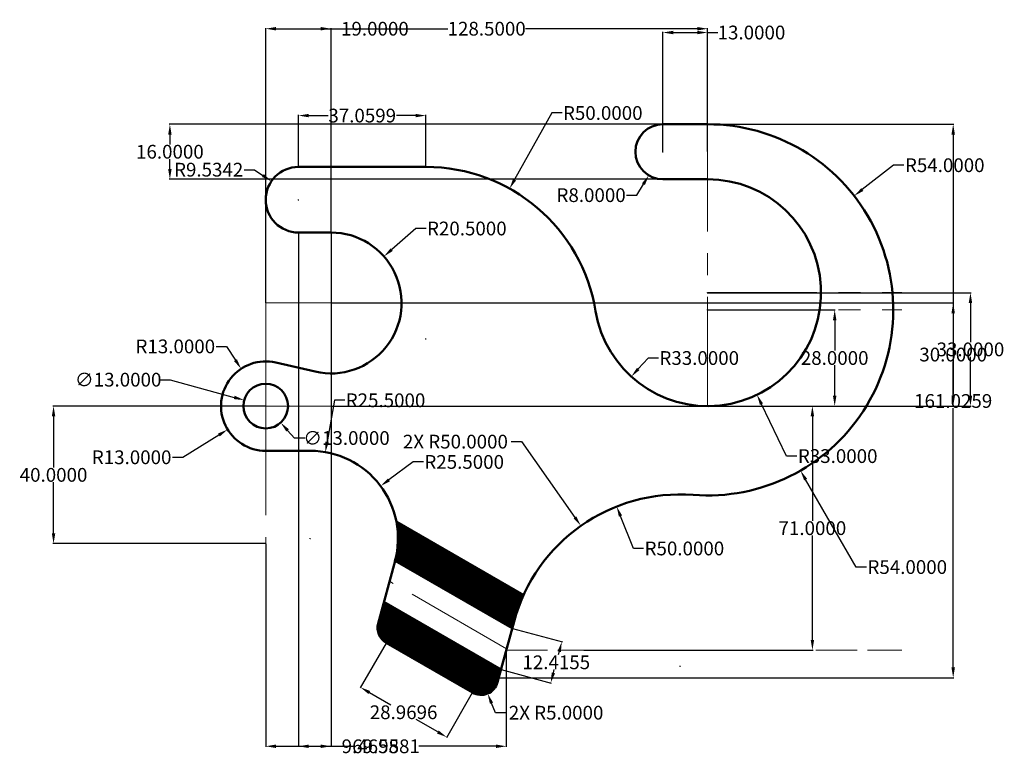
# Model space of a CAD drawing. Units: millimetres. Extents: x 855 to 1141, y 767 to 981.
import ezdxf

# ---------------------------------------------------------------- set-up
doc = ezdxf.new("R2010")
doc.units = ezdxf.units.MM
doc.header["$MEASUREMENT"] = 0
doc.linetypes.add('ACAD_ISO02W100', pattern=[15, 12, -3])
doc.linetypes.add('CENTER', pattern=[50.8, 31.75, -6.35, 6.35, -6.35])
for name, color, linetype, lineweight in [('M-CNTR', 55, 'CENTER', 18), ('M-CONS', 2, 'ACAD_ISO02W100', 13), ('M-DIMS', 2, 'Continuous', 25), ('M-HATC', 8, 'Continuous', 18), ('M-OUTL', 7, 'Continuous', 50)]:
    doc.layers.add(name, color=color, linetype=linetype, lineweight=lineweight)
doc.styles.get("Standard").update_dxf_attribs({"font": 'arial.ttf'})
doc.dimstyles.get("Standard").update_dxf_attribs({"dimtxt": 4, "dimasz": 3, "dimexe": 0.18, "dimexo": 0.0625, "dimgap": 0.09, "dimtad": 0, "dimtih": 1, "dimtoh": 1, "dimdec": 4, "dimzin": 0, "dimdsep": 46, "dimtxsty": 'Standard', "dimcen": 0.09, "dimadec": 0, "dimazin": 0, "dimtfac": 1, "dimtdec": 4, "dimtofl": 0, "dimtmove": 0, "dimatfit": 3, "dimfxl": 1, "dimtolj": 1, "dimtzin": 0, "dimarcsym": 0})

# ---------------------------------------------------------------- blocks, each defined once
blk = doc.blocks.new('*D1')
at = {"layer": 'Defpoints', "color": 0, "transparency": 16777216}
for p in [(1055.15, 901.49), (1032.96, 877.07)]:
    blk.add_point(p, dxfattribs=at)
at = {"layer": 'M-DIMS', "color": 0, "lineweight": -2, "transparency": 16777216}
for p, q in [((1037.87, 882.48), (1034.97, 879.29)), ((1040.87, 882.48), (1037.87, 882.48))]:
    blk.add_line(p, q, dxfattribs=at)
at = {"layer": 'M-DIMS', "color": 0, "transparency": 16777216}
blk.add_solid([(1034.6, 879.63), (1035.34, 878.96), (1032.96, 877.07)], dxfattribs=at)
at = {"layer": 'M-DIMS', "color": 0, "transparency": 16777216, "insert": (1052.72, 882.48), "char_height": 4, "attachment_point": 5}
blk.add_mtext('\\A1;R33.0000', dxfattribs=at)
blk = doc.blocks.new('*D2')
at = {"layer": 'Defpoints', "color": 0, "transparency": 16777216}
for p in [(997.56, 931.75), (973.24, 888.06)]:
    blk.add_point(p, dxfattribs=at)
at = {"layer": 'M-DIMS', "color": 0, "lineweight": -2, "transparency": 16777216}
for p, q in [((1009.81, 953.76), (999.02, 934.37)), ((1012.81, 953.76), (1009.81, 953.76)), ((973.15, 888.06), (973.33, 888.06)), ((973.24, 887.97), (973.24, 888.15))]:
    blk.add_line(p, q, dxfattribs=at)
at = {"layer": 'M-DIMS', "color": 0, "transparency": 16777216}
blk.add_solid([(998.58, 934.62), (999.46, 934.13), (997.56, 931.75)], dxfattribs=at)
at = {"layer": 'M-DIMS', "color": 0, "transparency": 16777216, "insert": (1024.66, 953.76), "char_height": 4, "attachment_point": 5}
blk.add_mtext('\\A1;R50.0000', dxfattribs=at)
blk = doc.blocks.new('*D3')
at = {"layer": 'Defpoints', "color": 0, "transparency": 16777216}
for p in [(1042.15, 942.49), (1038.03, 935.63)]:
    blk.add_point(p, dxfattribs=at)
at = {"layer": 'M-DIMS', "color": 0, "lineweight": -2, "transparency": 16777216}
for p, q in [((1042.06, 942.49), (1042.24, 942.49)), ((1042.15, 942.4), (1042.15, 942.58)), ((1034.57, 929.86), (1036.49, 933.06)), ((1031.57, 929.86), (1034.57, 929.86))]:
    blk.add_line(p, q, dxfattribs=at)
at = {"layer": 'M-DIMS', "color": 0, "transparency": 16777216}
blk.add_solid([(1036.06, 933.32), (1036.92, 932.8), (1038.03, 935.63)], dxfattribs=at)
at = {"layer": 'M-DIMS', "color": 0, "transparency": 16777216, "insert": (1021.27, 929.86), "char_height": 4, "attachment_point": 5}
blk.add_mtext('\\A1;R8.0000', dxfattribs=at)
blk = doc.blocks.new('*D4')
at = {"layer": 'Defpoints', "color": 0, "transparency": 16777216}
for p in [(926.65, 868.49), (915.58, 861.67)]:
    blk.add_point(p, dxfattribs=at)
at = {"layer": 'M-DIMS', "color": 0, "lineweight": -2, "transparency": 16777216}
for p, q in [((926.56, 868.49), (926.74, 868.49)), ((926.65, 868.4), (926.65, 868.58)), ((902.51, 853.61), (913.03, 860.1)), ((899.51, 853.61), (902.51, 853.61))]:
    blk.add_line(p, q, dxfattribs=at)
at = {"layer": 'M-DIMS', "color": 0, "transparency": 16777216}
blk.add_solid([(912.77, 860.52), (913.29, 859.67), (915.58, 861.67)], dxfattribs=at)
at = {"layer": 'M-DIMS', "color": 0, "transparency": 16777216, "insert": (887.66, 853.61), "char_height": 4, "attachment_point": 5}
blk.add_mtext('\\A1;R13.0000', dxfattribs=at)
blk = doc.blocks.new('*D5')
at = {"layer": 'Defpoints', "color": 0, "transparency": 16777216}
for p in [(920.39, 870.23), (932.92, 866.76)]:
    blk.add_point(p, dxfattribs=at)
at = {"layer": 'M-DIMS', "color": 0, "lineweight": -2, "transparency": 16777216}
for p, q in [((895.85, 876.18), (898.85, 876.18)), ((898.85, 876.18), (917.49, 871.03)), ((926.56, 868.49), (926.74, 868.49)), ((926.65, 868.4), (926.65, 868.58))]:
    blk.add_line(p, q, dxfattribs=at)
at = {"layer": 'M-DIMS', "color": 0, "transparency": 16777216}
blk.add_solid([(917.63, 871.51), (917.36, 870.54), (920.39, 870.23)], dxfattribs=at)
at = {"layer": 'M-DIMS', "color": 0, "transparency": 16777216, "insert": (883.74, 876.18), "char_height": 4, "attachment_point": 5}
blk.add_mtext('\\A1;∅13.0000', dxfattribs=at)
blk = doc.blocks.new('*D6')
at = {"layer": 'Defpoints', "color": 0, "transparency": 16777216}
for p in [(1028.71, 839.28), (1047.14, 792.8)]:
    blk.add_point(p, dxfattribs=at)
at = {"layer": 'M-DIMS', "color": 0, "lineweight": -2, "transparency": 16777216}
for p, q in [((1033.55, 827.08), (1029.82, 836.5)), ((1036.55, 827.08), (1033.55, 827.08))]:
    blk.add_line(p, q, dxfattribs=at)
at = {"layer": 'M-DIMS', "color": 0, "transparency": 16777216}
blk.add_solid([(1030.28, 836.68), (1029.35, 836.31), (1028.71, 839.28)], dxfattribs=at)
at = {"layer": 'M-DIMS', "color": 0, "transparency": 16777216, "insert": (1048.4, 827.08), "char_height": 4, "attachment_point": 5}
blk.add_mtext('\\A1;R50.0000', dxfattribs=at)
blk = doc.blocks.new('*D7')
at = {"layer": 'Defpoints', "color": 0, "transparency": 16777216}
for p in [(960.07, 845.22), (939.62, 829.99)]:
    blk.add_point(p, dxfattribs=at)
at = {"layer": 'M-DIMS', "color": 0, "lineweight": -2, "transparency": 16777216}
for p, q in [((969.51, 852.25), (962.48, 847.02)), ((972.51, 852.25), (969.51, 852.25)), ((939.53, 829.99), (939.71, 829.99)), ((939.62, 829.9), (939.62, 830.08))]:
    blk.add_line(p, q, dxfattribs=at)
at = {"layer": 'M-DIMS', "color": 0, "transparency": 16777216}
blk.add_solid([(962.18, 847.42), (962.77, 846.61), (960.07, 845.22)], dxfattribs=at)
at = {"layer": 'M-DIMS', "color": 0, "transparency": 16777216, "insert": (984.36, 852.25), "char_height": 4, "attachment_point": 5}
blk.add_mtext('\\A1;R25.5000', dxfattribs=at)
blk = doc.blocks.new('*D8')
at = {"layer": 'Defpoints', "color": 0, "transparency": 16777216}
for p in [(1055.15, 901.49), (1055.15, 868.49), (1131.58, 868.49)]:
    blk.add_point(p, dxfattribs=at)
at = {"layer": 'M-DIMS', "color": 0, "lineweight": -2, "transparency": 16777216}
for p, q in [((1055.21, 901.49), (1131.76, 901.49)), ((1131.58, 898.49), (1131.58, 887.13)), ((1131.58, 871.49), (1131.58, 882.86)), ((1055.21, 868.49), (1131.76, 868.49))]:
    blk.add_line(p, q, dxfattribs=at)
at = {"layer": 'M-DIMS', "color": 0, "transparency": 16777216}
for points in [[(1131.08, 898.49), (1132.08, 898.49), (1131.58, 901.49)], [(1131.08, 871.49), (1132.08, 871.49), (1131.58, 868.49)]]:
    blk.add_solid(points, dxfattribs=at)
at = {"layer": 'M-DIMS', "color": 0, "transparency": 16777216, "insert": (1131.58, 884.99), "char_height": 4, "attachment_point": 5}
blk.add_mtext('\\A1;33.0000', dxfattribs=at)
blk = doc.blocks.new('*D9')
at = {"layer": 'Defpoints', "color": 0, "transparency": 16777216}
for p in [(1055.15, 896.49), (1055.15, 868.49), (1092.1, 868.49)]:
    blk.add_point(p, dxfattribs=at)
at = {"layer": 'M-DIMS', "color": 0, "lineweight": -2, "transparency": 16777216}
for p, q in [((1055.21, 896.49), (1092.28, 896.49)), ((1092.1, 893.49), (1092.1, 884.63)), ((1092.1, 871.49), (1092.1, 880.36)), ((1055.21, 868.49), (1092.28, 868.49))]:
    blk.add_line(p, q, dxfattribs=at)
at = {"layer": 'M-DIMS', "color": 0, "transparency": 16777216}
for points in [[(1091.6, 893.49), (1092.6, 893.49), (1092.1, 896.49)], [(1091.6, 871.49), (1092.6, 871.49), (1092.1, 868.49)]]:
    blk.add_solid(points, dxfattribs=at)
at = {"layer": 'M-DIMS', "color": 0, "transparency": 16777216, "insert": (1092.1, 882.49), "char_height": 4, "attachment_point": 5}
blk.add_mtext('\\A1;28.0000', dxfattribs=at)
blk = doc.blocks.new('*D10')
at = {"layer": 'Defpoints', "color": 0, "transparency": 16777216}
for p in [(1097.78, 929.65), (1055.15, 896.49)]:
    blk.add_point(p, dxfattribs=at)
at = {"layer": 'M-DIMS', "color": 0, "lineweight": -2, "transparency": 16777216}
for p, q in [((1109.25, 938.57), (1100.14, 931.49)), ((1112.25, 938.57), (1109.25, 938.57)), ((1055.06, 896.49), (1055.24, 896.49)), ((1055.15, 896.4), (1055.15, 896.58))]:
    blk.add_line(p, q, dxfattribs=at)
at = {"layer": 'M-DIMS', "color": 0, "transparency": 16777216}
blk.add_solid([(1099.84, 931.88), (1100.45, 931.09), (1097.78, 929.65)], dxfattribs=at)
at = {"layer": 'M-DIMS', "color": 0, "transparency": 16777216, "insert": (1124.11, 938.57), "char_height": 4, "attachment_point": 5}
blk.add_mtext('\\A1;R54.0000', dxfattribs=at)
blk = doc.blocks.new('*D11')
at = {"layer": 'Defpoints', "color": 0, "transparency": 16777216}
for p in [(1055.15, 977.17), (1042.15, 942.49), (1055.15, 942.49)]:
    blk.add_point(p, dxfattribs=at)
at = {"layer": 'M-DIMS', "color": 0, "lineweight": -2, "transparency": 16777216}
for p, q in [((1042.15, 942.56), (1042.15, 977.35)), ((1045.15, 977.17), (1052.15, 977.17)), ((1055.15, 942.56), (1055.15, 977.35)), ((1055.15, 977.17), (1058.15, 977.17))]:
    blk.add_line(p, q, dxfattribs=at)
at = {"layer": 'M-DIMS', "color": 0, "transparency": 16777216}
for points in [[(1045.15, 977.67), (1045.15, 976.67), (1042.15, 977.17)], [(1052.15, 977.67), (1052.15, 976.67), (1055.15, 977.17)]]:
    blk.add_solid(points, dxfattribs=at)
at = {"layer": 'M-DIMS', "color": 0, "transparency": 16777216, "insert": (1067.9, 977.17), "char_height": 4, "attachment_point": 5}
blk.add_mtext('\\A1;13.0000', dxfattribs=at)
blk = doc.blocks.new('*D12')
at = {"layer": 'Defpoints', "color": 0, "transparency": 16777216}
for p in [(1019.13, 868.49), (1019.13, 797.49), (1085.62, 797.49)]:
    blk.add_point(p, dxfattribs=at)
at = {"layer": 'M-DIMS', "color": 0, "lineweight": -2, "transparency": 16777216}
for p, q in [((1019.19, 868.49), (1085.8, 868.49)), ((1085.62, 865.49), (1085.62, 835.13)), ((1085.62, 800.49), (1085.62, 830.86)), ((1019.19, 797.49), (1085.8, 797.49))]:
    blk.add_line(p, q, dxfattribs=at)
at = {"layer": 'M-DIMS', "color": 0, "transparency": 16777216}
for points in [[(1085.12, 865.49), (1086.12, 865.49), (1085.62, 868.49)], [(1085.12, 800.49), (1086.12, 800.49), (1085.62, 797.49)]]:
    blk.add_solid(points, dxfattribs=at)
at = {"layer": 'M-DIMS', "color": 0, "transparency": 16777216, "insert": (1085.62, 832.99), "char_height": 4, "attachment_point": 5}
blk.add_mtext('\\A1;71.0000', dxfattribs=at)
blk = doc.blocks.new('*D13')
at = {"layer": 'Defpoints', "color": 0, "transparency": 16777216}
for p in [(926.74, 868.49), (864.95, 828.49), (926.65, 828.49)]:
    blk.add_point(p, dxfattribs=at)
at = {"layer": 'M-DIMS', "color": 0, "lineweight": -2, "transparency": 16777216}
for p, q in [((926.68, 868.49), (864.77, 868.49)), ((864.95, 865.49), (864.95, 850.63)), ((864.95, 831.49), (864.95, 846.36)), ((926.59, 828.49), (864.77, 828.49))]:
    blk.add_line(p, q, dxfattribs=at)
at = {"layer": 'M-DIMS', "color": 0, "transparency": 16777216}
for points in [[(864.45, 865.49), (865.45, 865.49), (864.95, 868.49)], [(864.45, 831.49), (865.45, 831.49), (864.95, 828.49)]]:
    blk.add_solid(points, dxfattribs=at)
at = {"layer": 'M-DIMS', "color": 0, "transparency": 16777216, "insert": (864.95, 848.49), "char_height": 4, "attachment_point": 5}
blk.add_mtext('\\A1;40.0000', dxfattribs=at)
blk = doc.blocks.new('*D14')
at = {"layer": 'Defpoints', "color": 0, "transparency": 16777216}
for p in [(1055.15, 978.28), (1055.15, 950.49), (926.65, 898.49)]:
    blk.add_point(p, dxfattribs=at)
at = {"layer": 'M-DIMS', "color": 0, "lineweight": -2, "transparency": 16777216}
for p, q in [((926.65, 898.56), (926.65, 978.46)), ((929.65, 978.28), (979.59, 978.28)), ((1052.15, 978.28), (1002.21, 978.28)), ((1055.15, 950.56), (1055.15, 978.46))]:
    blk.add_line(p, q, dxfattribs=at)
at = {"layer": 'M-DIMS', "color": 0, "transparency": 16777216}
for points in [[(929.65, 978.78), (929.65, 977.78), (926.65, 978.28)], [(1052.15, 978.78), (1052.15, 977.78), (1055.15, 978.28)]]:
    blk.add_solid(points, dxfattribs=at)
at = {"layer": 'M-DIMS', "color": 0, "transparency": 16777216, "insert": (990.9, 978.28), "char_height": 4, "attachment_point": 5}
blk.add_mtext('\\A1;128.5000', dxfattribs=at)
blk = doc.blocks.new('*D15')
at = {"layer": 'Defpoints', "color": 0, "transparency": 16777216}
for p in [(1055.15, 950.49), (1126.56, 950.49), (989.26, 789.47)]:
    blk.add_point(p, dxfattribs=at)
at = {"layer": 'M-DIMS', "color": 0, "lineweight": -2, "transparency": 16777216}
for p, q in [((1055.21, 950.49), (1126.74, 950.49)), ((1126.56, 947.49), (1126.56, 872.11)), ((1126.56, 792.47), (1126.56, 867.85)), ((989.32, 789.47), (1126.74, 789.47))]:
    blk.add_line(p, q, dxfattribs=at)
at = {"layer": 'M-DIMS', "color": 0, "transparency": 16777216}
for points in [[(1126.06, 947.49), (1127.06, 947.49), (1126.56, 950.49)], [(1126.06, 792.47), (1127.06, 792.47), (1126.56, 789.47)]]:
    blk.add_solid(points, dxfattribs=at)
at = {"layer": 'M-DIMS', "color": 0, "transparency": 16777216, "insert": (1126.56, 869.98), "char_height": 4, "attachment_point": 5}
blk.add_mtext('\\A1;161.0259', dxfattribs=at)
blk = doc.blocks.new('*D16')
at = {"layer": 'Defpoints', "color": 0, "transparency": 16777216}
for p in [(945.65, 978.28), (945.65, 918.99), (926.65, 898.49)]:
    blk.add_point(p, dxfattribs=at)
at = {"layer": 'M-DIMS', "color": 0, "lineweight": -2, "transparency": 16777216}
for p, q in [((926.65, 898.56), (926.65, 978.46)), ((929.65, 978.28), (942.65, 978.28)), ((945.65, 919.06), (945.65, 978.46)), ((945.65, 978.28), (948.65, 978.28))]:
    blk.add_line(p, q, dxfattribs=at)
at = {"layer": 'M-DIMS', "color": 0, "transparency": 16777216}
for points in [[(929.65, 978.78), (929.65, 977.78), (926.65, 978.28)], [(942.65, 978.78), (942.65, 977.78), (945.65, 978.28)]]:
    blk.add_solid(points, dxfattribs=at)
at = {"layer": 'M-DIMS', "color": 0, "transparency": 16777216, "insert": (958.4, 978.28), "char_height": 4, "attachment_point": 5}
blk.add_mtext('\\A1;19.0000', dxfattribs=at)
blk = doc.blocks.new('*D17')
at = {"layer": 'Defpoints', "color": 0, "transparency": 16777216}
for p in [(945.65, 898.49), (1126.56, 898.49), (945.65, 868.49)]:
    blk.add_point(p, dxfattribs=at)
at = {"layer": 'M-DIMS', "color": 0, "lineweight": -2, "transparency": 16777216}
for p, q in [((945.71, 898.49), (1126.74, 898.49)), ((1126.56, 895.49), (1126.56, 885.63)), ((1126.56, 871.49), (1126.56, 881.36)), ((945.71, 868.49), (1126.74, 868.49))]:
    blk.add_line(p, q, dxfattribs=at)
at = {"layer": 'M-DIMS', "color": 0, "transparency": 16777216}
for points in [[(1126.06, 895.49), (1127.06, 895.49), (1126.56, 898.49)], [(1126.06, 871.49), (1127.06, 871.49), (1126.56, 868.49)]]:
    blk.add_solid(points, dxfattribs=at)
at = {"layer": 'M-DIMS', "color": 0, "transparency": 16777216, "insert": (1126.56, 883.49), "char_height": 4, "attachment_point": 5}
blk.add_mtext('\\A1;30.0000', dxfattribs=at)
blk = doc.blocks.new('*D18')
at = {"layer": 'Defpoints', "color": 0, "transparency": 16777216}
for p in [(898.78, 950.49), (1042.15, 950.49), (1042.15, 934.49)]:
    blk.add_point(p, dxfattribs=at)
at = {"layer": 'M-DIMS', "color": 0, "lineweight": -2, "transparency": 16777216}
for p, q in [((1042.09, 950.49), (898.6, 950.49)), ((898.78, 947.49), (898.78, 944.63)), ((898.78, 937.49), (898.78, 940.36)), ((1042.09, 934.49), (898.6, 934.49))]:
    blk.add_line(p, q, dxfattribs=at)
at = {"layer": 'M-DIMS', "color": 0, "transparency": 16777216}
for points in [[(898.28, 947.49), (899.28, 947.49), (898.78, 950.49)], [(898.28, 937.49), (899.28, 937.49), (898.78, 934.49)]]:
    blk.add_solid(points, dxfattribs=at)
at = {"layer": 'M-DIMS', "color": 0, "transparency": 16777216, "insert": (898.78, 942.49), "char_height": 4, "attachment_point": 5}
blk.add_mtext('\\A1;16.0000', dxfattribs=at)
blk = doc.blocks.new('*D19')
at = {"layer": 'Defpoints', "color": 0, "transparency": 16777216}
for p in [(961.67, 799.62), (954.19, 786.68), (986.76, 785.14)]:
    blk.add_point(p, dxfattribs=at)
at = {"layer": 'M-DIMS', "color": 0, "lineweight": -2, "transparency": 16777216}
for p, q in [((961.64, 799.57), (954.1, 786.52)), ((956.79, 785.18), (963.05, 781.57)), ((986.73, 785.08), (979.19, 772.03)), ((976.69, 773.69), (970.43, 777.3))]:
    blk.add_line(p, q, dxfattribs=at)
at = {"layer": 'M-DIMS', "color": 0, "transparency": 16777216}
for points in [[(957.04, 785.61), (956.54, 784.74), (954.19, 786.68)], [(976.94, 774.12), (976.44, 773.26), (979.28, 772.19)]]:
    blk.add_solid(points, dxfattribs=at)
at = {"layer": 'M-DIMS', "color": 0, "transparency": 16777216, "insert": (966.74, 779.43), "char_height": 4, "attachment_point": 5}
blk.add_mtext('\\A1;28.9696', dxfattribs=at)
blk = doc.blocks.new('*D20')
at = {"layer": 'Defpoints', "color": 0, "transparency": 16777216}
for p in [(926.65, 828.49), (996.61, 797.49), (996.61, 769.53)]:
    blk.add_point(p, dxfattribs=at)
at = {"layer": 'M-DIMS', "color": 0, "lineweight": -2, "transparency": 16777216}
for p, q in [((926.65, 828.43), (926.65, 769.35)), ((996.61, 797.43), (996.61, 769.35)), ((929.65, 769.53), (952.06, 769.53)), ((993.61, 769.53), (971.2, 769.53))]:
    blk.add_line(p, q, dxfattribs=at)
at = {"layer": 'M-DIMS', "color": 0, "transparency": 16777216}
for points in [[(929.65, 770.03), (929.65, 769.03), (926.65, 769.53)], [(993.61, 770.03), (993.61, 769.03), (996.61, 769.53)]]:
    blk.add_solid(points, dxfattribs=at)
at = {"layer": 'M-DIMS', "color": 0, "transparency": 16777216, "insert": (961.63, 769.53), "char_height": 4, "attachment_point": 5}
blk.add_mtext('\\A1;69.9581', dxfattribs=at)
blk = doc.blocks.new('*D21')
at = {"layer": 'Defpoints', "color": 0, "transparency": 16777216}
for p in [(973.24, 953.01), (936.18, 938.06), (973.24, 938.06)]:
    blk.add_point(p, dxfattribs=at)
at = {"layer": 'M-DIMS', "color": 0, "lineweight": -2, "transparency": 16777216}
for p, q in [((936.18, 938.12), (936.18, 953.19)), ((939.18, 953.01), (944.77, 953.01)), ((970.24, 953.01), (964.66, 953.01)), ((973.24, 938.12), (973.24, 953.19))]:
    blk.add_line(p, q, dxfattribs=at)
at = {"layer": 'M-DIMS', "color": 0, "transparency": 16777216}
for points in [[(939.18, 953.51), (939.18, 952.51), (936.18, 953.01)], [(970.24, 953.51), (970.24, 952.51), (973.24, 953.01)]]:
    blk.add_solid(points, dxfattribs=at)
at = {"layer": 'M-DIMS', "color": 0, "transparency": 16777216, "insert": (954.71, 953.01), "char_height": 4, "attachment_point": 5}
blk.add_mtext('\\A1;37.0599', dxfattribs=at)
blk = doc.blocks.new('*D22')
at = {"layer": 'Defpoints', "color": 0, "transparency": 16777216}
for p in [(936.18, 918.99), (945.65, 918.99), (945.65, 769.53)]:
    blk.add_point(p, dxfattribs=at)
at = {"layer": 'M-DIMS', "color": 0, "lineweight": -2, "transparency": 16777216}
for p, q in [((936.18, 918.93), (936.18, 769.35)), ((945.65, 918.93), (945.65, 769.35)), ((939.18, 769.53), (942.65, 769.53)), ((945.65, 769.53), (948.65, 769.53))]:
    blk.add_line(p, q, dxfattribs=at)
at = {"layer": 'M-DIMS', "color": 0, "transparency": 16777216}
for points in [[(939.18, 770.03), (939.18, 769.03), (936.18, 769.53)], [(942.65, 770.03), (942.65, 769.03), (945.65, 769.53)]]:
    blk.add_solid(points, dxfattribs=at)
at = {"layer": 'M-DIMS', "color": 0, "transparency": 16777216, "insert": (957.05, 769.53), "char_height": 4, "attachment_point": 5}
blk.add_mtext('\\A1;9.4658', dxfattribs=at)
blk = doc.blocks.new('*D23')
at = {"layer": 'Defpoints', "color": 0, "transparency": 16777216}
for p in [(998.33, 803.86), (995.09, 791.88), (1009.52, 787.97)]:
    blk.add_point(p, dxfattribs=at)
at = {"layer": 'M-DIMS', "color": 0, "lineweight": -2, "transparency": 16777216}
for p, q in [((998.39, 803.84), (1012.94, 799.91)), ((1011.98, 797.06), (1011.72, 796.1)), ((995.15, 791.86), (1009.69, 787.92)), ((1010.3, 790.87), (1010.56, 791.83))]:
    blk.add_line(p, q, dxfattribs=at)
at = {"layer": 'M-DIMS', "color": 0, "transparency": 16777216}
for points in [[(1011.5, 797.19), (1012.46, 796.93), (1012.76, 799.96)], [(1009.82, 791), (1010.79, 790.74), (1009.52, 787.97)]]:
    blk.add_solid(points, dxfattribs=at)
at = {"layer": 'M-DIMS', "color": 0, "transparency": 16777216, "insert": (1011.14, 793.96), "char_height": 4, "attachment_point": 5}
blk.add_mtext('\\A1;12.4155', dxfattribs=at)
blk = doc.blocks.new('*D24')
at = {"layer": 'Defpoints', "color": 0, "transparency": 16777216}
for p in [(1055.15, 896.49), (1082.15, 849.73)]:
    blk.add_point(p, dxfattribs=at)
at = {"layer": 'M-DIMS', "color": 0, "lineweight": -2, "transparency": 16777216}
for p, q in [((1055.06, 896.49), (1055.24, 896.49)), ((1055.15, 896.4), (1055.15, 896.58)), ((1098.35, 821.67), (1083.65, 847.13)), ((1101.35, 821.67), (1098.35, 821.67))]:
    blk.add_line(p, q, dxfattribs=at)
at = {"layer": 'M-DIMS', "color": 0, "transparency": 16777216}
blk.add_solid([(1084.08, 847.38), (1083.22, 846.88), (1082.15, 849.73)], dxfattribs=at)
at = {"layer": 'M-DIMS', "color": 0, "transparency": 16777216, "insert": (1113.21, 821.67), "char_height": 4, "attachment_point": 5}
blk.add_mtext('\\A1;R54.0000', dxfattribs=at)
blk = doc.blocks.new('*D25')
at = {"layer": 'Defpoints', "color": 0, "transparency": 16777216}
for p in [(1018.3, 833.65), (1047.14, 792.8)]:
    blk.add_point(p, dxfattribs=at)
at = {"layer": 'M-DIMS', "color": 0, "lineweight": -2, "transparency": 16777216}
for p, q in [((998, 858.16), (1001, 858.16)), ((1001, 858.16), (1016.57, 836.1)), ((1047.05, 792.8), (1047.23, 792.8)), ((1047.14, 792.71), (1047.14, 792.89))]:
    blk.add_line(p, q, dxfattribs=at)
at = {"layer": 'M-DIMS', "color": 0, "transparency": 16777216}
blk.add_solid([(1016.98, 836.39), (1016.16, 835.81), (1018.3, 833.65)], dxfattribs=at)
at = {"layer": 'M-DIMS', "color": 0, "transparency": 16777216, "insert": (981.81, 858.16), "char_height": 4, "attachment_point": 5}
blk.add_mtext('\\A1;2X R50.0000', dxfattribs=at)
blk = doc.blocks.new('*D26')
at = {"layer": 'Defpoints', "color": 0, "transparency": 16777216}
for p in [(1055.15, 901.49), (1069.51, 871.78)]:
    blk.add_point(p, dxfattribs=at)
at = {"layer": 'M-DIMS', "color": 0, "lineweight": -2, "transparency": 16777216}
for p, q in [((1055.06, 901.49), (1055.24, 901.49)), ((1055.15, 901.4), (1055.15, 901.58)), ((1078.12, 853.95), (1070.81, 869.08)), ((1081.12, 853.95), (1078.12, 853.95))]:
    blk.add_line(p, q, dxfattribs=at)
at = {"layer": 'M-DIMS', "color": 0, "transparency": 16777216}
blk.add_solid([(1071.26, 869.3), (1070.36, 868.86), (1069.51, 871.78)], dxfattribs=at)
at = {"layer": 'M-DIMS', "color": 0, "transparency": 16777216, "insert": (1092.98, 853.95), "char_height": 4, "attachment_point": 5}
blk.add_mtext('\\A1;R33.0000', dxfattribs=at)
blk = doc.blocks.new('*D27')
at = {"layer": 'Defpoints', "color": 0, "transparency": 16777216}
for p in [(944, 855.11), (939.62, 829.99)]:
    blk.add_point(p, dxfattribs=at)
at = {"layer": 'M-DIMS', "color": 0, "lineweight": -2, "transparency": 16777216}
for p, q in [((946.63, 870.19), (944.52, 858.07)), ((949.63, 870.19), (946.63, 870.19)), ((939.53, 829.99), (939.71, 829.99)), ((939.62, 829.9), (939.62, 830.08))]:
    blk.add_line(p, q, dxfattribs=at)
at = {"layer": 'M-DIMS', "color": 0, "transparency": 16777216}
blk.add_solid([(944.03, 858.16), (945.01, 857.98), (944, 855.11)], dxfattribs=at)
at = {"layer": 'M-DIMS', "color": 0, "transparency": 16777216, "insert": (961.49, 870.19), "char_height": 4, "attachment_point": 5}
blk.add_mtext('\\A1;R25.5000', dxfattribs=at)
blk = doc.blocks.new('*D28')
at = {"layer": 'Defpoints', "color": 0, "transparency": 16777216}
for p in [(961.04, 912.04), (945.65, 898.49)]:
    blk.add_point(p, dxfattribs=at)
at = {"layer": 'M-DIMS', "color": 0, "lineweight": -2, "transparency": 16777216}
for p, q in [((970.27, 920.16), (963.29, 914.02)), ((973.27, 920.16), (970.27, 920.16)), ((945.56, 898.49), (945.74, 898.49)), ((945.65, 898.4), (945.65, 898.58))]:
    blk.add_line(p, q, dxfattribs=at)
at = {"layer": 'M-DIMS', "color": 0, "transparency": 16777216}
blk.add_solid([(962.96, 914.39), (963.62, 913.64), (961.04, 912.04)], dxfattribs=at)
at = {"layer": 'M-DIMS', "color": 0, "transparency": 16777216, "insert": (985.13, 920.16), "char_height": 4, "attachment_point": 5}
blk.add_mtext('\\A1;R20.5000', dxfattribs=at)
blk = doc.blocks.new('*D29')
at = {"layer": 'Defpoints', "color": 0, "transparency": 16777216}
for p in [(919.5, 879.35), (926.65, 868.49)]:
    blk.add_point(p, dxfattribs=at)
at = {"layer": 'M-DIMS', "color": 0, "lineweight": -2, "transparency": 16777216}
for p, q in [((912.21, 885.86), (915.21, 885.86)), ((915.21, 885.86), (917.85, 881.86)), ((926.56, 868.49), (926.74, 868.49)), ((926.65, 868.4), (926.65, 868.58))]:
    blk.add_line(p, q, dxfattribs=at)
at = {"layer": 'M-DIMS', "color": 0, "transparency": 16777216}
blk.add_solid([(918.27, 882.13), (917.43, 881.58), (919.5, 879.35)], dxfattribs=at)
at = {"layer": 'M-DIMS', "color": 0, "transparency": 16777216, "insert": (900.36, 885.86), "char_height": 4, "attachment_point": 5}
blk.add_mtext('\\A1;R13.0000', dxfattribs=at)
blk = doc.blocks.new('*D30')
at = {"layer": 'Defpoints', "color": 0, "transparency": 16777216}
for p in [(928.31, 933.9), (936.18, 928.53)]:
    blk.add_point(p, dxfattribs=at)
at = {"layer": 'M-DIMS', "color": 0, "lineweight": -2, "transparency": 16777216}
for p, q in [((920.35, 937.27), (923.35, 937.27)), ((923.35, 937.27), (925.83, 935.59)), ((936.09, 928.53), (936.27, 928.53)), ((936.18, 928.44), (936.18, 928.62))]:
    blk.add_line(p, q, dxfattribs=at)
at = {"layer": 'M-DIMS', "color": 0, "transparency": 16777216}
blk.add_solid([(926.11, 936), (925.54, 935.17), (928.31, 933.9)], dxfattribs=at)
at = {"layer": 'M-DIMS', "color": 0, "transparency": 16777216, "insert": (910.06, 937.27), "char_height": 4, "attachment_point": 5}
blk.add_mtext('\\A1;R9.5342', dxfattribs=at)
blk = doc.blocks.new('*D31')
at = {"layer": 'Defpoints', "color": 0, "transparency": 16777216}
for p in [(922.3, 873.32), (931, 863.67)]:
    blk.add_point(p, dxfattribs=at)
at = {"layer": 'M-DIMS', "color": 0, "lineweight": -2, "transparency": 16777216}
for p, q in [((926.56, 868.49), (926.74, 868.49)), ((926.65, 868.4), (926.65, 868.58)), ((935.02, 859.21), (933.01, 861.44)), ((938.02, 859.21), (935.02, 859.21))]:
    blk.add_line(p, q, dxfattribs=at)
at = {"layer": 'M-DIMS', "color": 0, "transparency": 16777216}
blk.add_solid([(933.38, 861.77), (932.64, 861.1), (931, 863.67)], dxfattribs=at)
at = {"layer": 'M-DIMS', "color": 0, "transparency": 16777216, "insert": (950.14, 859.21), "char_height": 4, "attachment_point": 5}
blk.add_mtext('\\A1;∅13.0000', dxfattribs=at)
blk = doc.blocks.new('*D32')
at = {"layer": 'Defpoints', "color": 0, "transparency": 16777216}
for p in [(989.26, 789.47), (991.17, 784.85)]:
    blk.add_point(p, dxfattribs=at)
at = {"layer": 'M-DIMS', "color": 0, "lineweight": -2, "transparency": 16777216}
for p, q in [((989.17, 789.47), (989.35, 789.47)), ((989.26, 789.38), (989.26, 789.56)), ((993.46, 779.3), (992.31, 782.07)), ((996.46, 779.3), (993.46, 779.3))]:
    blk.add_line(p, q, dxfattribs=at)
at = {"layer": 'M-DIMS', "color": 0, "transparency": 16777216}
blk.add_solid([(992.77, 782.26), (991.85, 781.88), (991.17, 784.85)], dxfattribs=at)
at = {"layer": 'M-DIMS', "color": 0, "transparency": 16777216, "insert": (1011.09, 779.3), "char_height": 4, "attachment_point": 5}
blk.add_mtext('\\A1;2X R5.0000', dxfattribs=at)

msp = doc.modelspace()

# ---------------------------------------------------------------- hatches: boundary and pattern name
at = {"layer": 'M-HATC'}
h = msp.add_hatch(dxfattribs=at)
h.set_pattern_fill('ANSI32', color=256)
h.paths.add_polyline_path([(961.04045, 811.53293), (959.3433, 805.2581, 0.340109602), (961.66987, 799.62253), (986.75826, 785.13774, 0.492415245), (994.08483, 788.16243), (995.08897, 791.87501)])
h.paths.add_polyline_path([(964.65016, 834.85228, -0.112586578), (964.28137, 823.51819), (998.33052, 803.8599), (998.87078, 805.85738, -0.040710067), (1001.62384, 813.50551)])

# ---------------------------------------------------------------- linework, layer by layer
at = {"layer": 'M-CNTR'}
for p, q in [((1055.15054, 868.49374), (1055.15054, 963.3315)), ((926.65054, 868.49374), (926.65054, 902.51976)), ((1055.15054, 901.49374), (1111.60941, 901.49374)), ((926.65054, 898.49374), (1111.60941, 898.49374)), ((945.65054, 868.49374), (945.65054, 898.49374)), ((1055.15054, 896.49374), (1111.60941, 896.49374)), ((926.65054, 868.49374), (1111.60941, 868.49374)), ((926.65054, 868.49374), (926.65054, 828.49374)), ((996.70975, 797.86746), (962.66122, 817.52538))]:
    msp.add_line(p, q, dxfattribs=at)
at = {"layer": 'M-CONS'}
msp.add_line((996.60867, 797.49374), (1111.60941, 797.49374), dxfattribs=at)
at = {"layer": 'M-OUTL'}
for p, q in [((1055.15054, 950.49374), (1042.15054, 950.49374)), ((973.24456, 938.06205), (936.1847, 938.06205)), ((1055.15054, 934.49374), (1042.15054, 934.49374)), ((945.65054, 918.99374), (936.1847, 918.99374)), ((929.56934, 881.16183), (941.04782, 878.51713)), ((926.65054, 855.49374), (939.61729, 855.49374)), ((1001.62384, 813.50551), (964.65016, 834.85228)), ((964.282, 823.51783), (959.3433, 805.2581)), ((998.33052, 803.8599), (964.282, 823.51783)), ((995.08897, 791.87501), (961.04045, 811.53293)), ((998.87078, 805.85739), (994.08483, 788.16243)), ((986.75826, 785.13774), (961.66987, 799.62253))]:
    msp.add_line(p, q, dxfattribs=at)
msp.add_circle((926.65054, 868.49374), 6.5, dxfattribs=at)
for centre, radius, start, end in [((1042.15054, 942.49374), 8, 90, 270), ((1055.15054, 896.49374), 54, 265.5805288, 90), ((936.1847, 928.52789), 9.53416, 90, 270), ((973.24456, 888.06205), 50, 9.3129909, 90), ((1055.15054, 901.49374), 33, 189.3129909, 90), ((945.65054, 898.49374), 20.5, 257.0251729, 90), ((926.65054, 868.49374), 13, 77.0251729, 270), ((939.61729, 829.99374), 25.5, 344.8653518, 90), ((1047.13652, 792.80297), 50, 85.5805288, 164.8653518), ((964.16987, 803.95265), 5, 164.8653518, 240), ((989.25826, 789.46787), 5, 240, 344.8653518)]:
    msp.add_arc(centre, radius, start, end, dxfattribs=at)

# ---------------------------------------------------------------- dimensions: what is measured, and where the dimension line sits
at = {"layer": 'M-DIMS'}
for base, p1, p2, override, picture, middle in [((1055.15054, 978.2815), (926.65054, 898.49374), (1055.15054, 950.49374), {"dimdec": 4, "dimlfac": 1, "dimrnd": 0, "dimzin": 0, "dimdsep": 46, "dimlunit": 2}, '*D14', (990.90054, 978.2815)), ((945.65054, 978.2815), (926.65054, 898.49374), (945.65054, 918.99374), {"dimdec": 4, "dimlfac": 1, "dimrnd": 0, "dimzin": 0, "dimdsep": 46, "dimlunit": 2}, '*D16', (958.40221, 978.2815)), ((1055.15054, 977.16547), (1042.15054, 942.49374), (1055.15054, 942.49374), {"dimclrd": 0, "dimclre": 0, "dimclrt": 0}, '*D11', (1067.90221, 977.16547)), ((973.24456, 953.01205), (936.1847, 938.06205), (973.24456, 938.06205), {"dimdec": 4, "dimlfac": 1, "dimrnd": 0, "dimzin": 0, "dimdsep": 46, "dimlunit": 2}, '*D21', (954.71463, 953.01205)), ((945.65054, 769.52877), (936.1847, 918.99374), (945.65054, 918.99374), {"dimdec": 4, "dimlfac": 1, "dimrnd": 0, "dimzin": 0, "dimdsep": 46, "dimlunit": 2}, '*D22', (957.0475, 769.52877)), ((996.60867, 769.52877), (926.65054, 828.49374), (996.60867, 797.49374), {"dimdec": 4, "dimlfac": 1, "dimrnd": 0, "dimzin": 0, "dimdsep": 46, "dimlunit": 2}, '*D20', (961.6296, 769.52877))]:
    dim = msp.add_linear_dim(base=base, p1=p1, p2=p2, dimstyle='Standard', override=override, dxfattribs=at)
    dim.commit()
    dim.dimension.update_dxf_attribs({"geometry": picture, "text_midpoint": middle})
for center, mpoint, override, picture, middle in [((973.24456, 888.06205), (997.56116, 931.75075), {"dimclrd": 0, "dimclre": 0, "dimclrt": 0}, '*D2', (1024.66497, 953.75954)), ((1042.15054, 942.49374), (1038.03342, 935.63449), {"dimclrd": 0, "dimclre": 0, "dimclrt": 0}, '*D3', (1021.26871, 929.86234)), ((1055.15054, 896.49374), (1097.77603, 929.64594), {"dimclrd": 0, "dimclre": 0, "dimclrt": 0}, '*D10', (1124.10561, 938.57115)), ((945.65054, 898.49374), (961.0408, 912.0359), {"dimdec": 4, "dimlfac": 1, "dimrnd": 0, "dimzin": 0, "dimdsep": 46, "dimlunit": 2}, '*D28', (985.12893, 920.16119)), ((1055.15054, 901.49374), (1032.95553, 877.07282), {"dimclrd": 0, "dimclre": 0, "dimclrt": 0}, '*D1', (1052.72382, 882.47997)), ((1055.15054, 901.49374), (1069.50907, 871.78124), {"dimdec": 4, "dimlfac": 1, "dimrnd": 0, "dimzin": 0, "dimdsep": 46, "dimlunit": 2}, '*D26', (1092.97817, 853.95374)), ((1055.15054, 896.49374), (1082.15084, 849.72854), {"dimdec": 4, "dimlfac": 1, "dimrnd": 0, "dimzin": 0, "dimdsep": 46, "dimlunit": 2}, '*D24', (1113.20501, 821.66942)), ((926.65054, 868.49374), (919.49976, 879.35036), {"dimdec": 4, "dimlfac": 1, "dimrnd": 0, "dimzin": 0, "dimdsep": 46, "dimlunit": 2}, '*D29', (900.35531, 885.86434)), ((939.61729, 829.99374), (944.00242, 855.11386), {"dimdec": 4, "dimlfac": 1, "dimrnd": 0, "dimzin": 0, "dimdsep": 46, "dimlunit": 2}, '*D27', (961.48748, 870.18594)), ((926.65054, 868.49374), (915.5845, 861.67151), {"dimclrd": 0, "dimclre": 0, "dimclrt": 0}, '*D4', (887.65741, 853.61192)), ((939.61729, 829.99374), (960.06979, 845.22349), {"dimclrd": 0, "dimclre": 0, "dimclrt": 0}, '*D7', (984.35983, 852.24996)), ((1047.13652, 792.80297), (1028.71268, 839.28481), {"dimclrd": 0, "dimclre": 0, "dimclrt": 0}, '*D6', (1048.40301, 827.08311))]:
    dim = msp.add_radius_dim(center=center, mpoint=mpoint, dimstyle='Standard', override=override, dxfattribs=at)
    dim.commit()
    dim.dimension.update_dxf_attribs({"geometry": picture, "text_midpoint": middle, "dimtype": 164})
for base, p1, p2, angle, override, picture, middle in [((898.78379, 950.49374), (1042.15054, 934.49374), (1042.15054, 950.49374), 90, {"dimdec": 4, "dimlfac": 1, "dimrnd": 0, "dimzin": 0, "dimdsep": 46, "dimlunit": 2}, '*D18', (898.78379, 942.49374)), ((1126.55941, 950.49374), (989.25826, 789.46787), (1055.15054, 950.49374), 90, {"dimdec": 4, "dimlfac": 1, "dimrnd": 0, "dimzin": 0, "dimdsep": 46, "dimlunit": 2}, '*D15', (1126.55941, 869.9808)), ((1131.58281, 868.49374), (1055.15054, 901.49374), (1055.15054, 868.49374), 90, {"dimclrd": 0, "dimclre": 0, "dimclrt": 0}, '*D8', (1131.58281, 884.99374)), ((1126.55941, 898.49374), (945.65054, 868.49374), (945.65054, 898.49374), 90, {"dimdec": 4, "dimlfac": 1, "dimrnd": 0, "dimzin": 0, "dimdsep": 46, "dimlunit": 2}, '*D17', (1126.55941, 883.49374)), ((1092.09612, 868.49374), (1055.15054, 896.49374), (1055.15054, 868.49374), 90, {"dimclrd": 0, "dimclre": 0, "dimclrt": 0}, '*D9', (1092.09612, 882.49374)), ((864.94866, 828.49374), (926.74054, 868.49374), (926.65054, 828.49374), 90, {"dimclrd": 0, "dimclre": 0, "dimclrt": 0}, '*D13', (864.94866, 848.49374)), ((1085.6243, 797.49374), (1019.12998, 868.49374), (1019.12998, 797.49374), 90, {"dimclrd": 0, "dimclre": 0, "dimclrt": 0}, '*D12', (1085.6243, 832.99374)), ((1009.52043, 787.97174), (998.33052, 803.8599), (995.08897, 791.87501), 254.8653518, {"dimdec": 4, "dimlfac": 1, "dimrnd": 0, "dimzin": 0, "dimdsep": 46, "dimlunit": 2}, '*D23', (1011.1412, 793.96419)), ((954.19487, 786.67545), (986.75826, 785.13774), (961.66987, 799.62253), 150, {"dimdec": 4, "dimlfac": 1, "dimrnd": 0, "dimzin": 0, "dimdsep": 46, "dimlunit": 2}, '*D19', (966.73906, 779.43306))]:
    dim = msp.add_linear_dim(base=base, p1=p1, p2=p2, angle=angle, dimstyle='Standard', override=override, dxfattribs=at)
    dim.commit()
    dim.dimension.update_dxf_attribs({"geometry": picture, "text_midpoint": middle})
dim = msp.add_radius_dim(center=(936.1847, 928.52789), mpoint=(928.30554, 933.89623), dimstyle='Standard', override={"dimdec": 4, "dimlfac": 1, "dimrnd": 0, "dimzin": 0, "dimdsep": 46, "dimlunit": 2}, dxfattribs=at)
dim.commit()
dim.dimension.update_dxf_attribs({"geometry": '*D30', "text_midpoint": (910.0606, 937.27461)})
for p1, p2, override, picture, middle in [((932.91553, 866.7617), (920.38556, 870.22578), {"dimclrd": 0, "dimclre": 0, "dimclrt": 0}, '*D5', (883.73587, 876.17908)), ((922.2978, 873.32112), (931.00329, 863.66636), {"dimdec": 4, "dimlfac": 1, "dimrnd": 0, "dimzin": 0, "dimdsep": 46, "dimlunit": 2}, '*D31', (950.13712, 859.21031))]:
    dim = msp.add_diameter_dim_2p(p1=p1, p2=p2, dimstyle='Standard', override=override, dxfattribs=at)
    dim.commit()
    dim.dimension.update_dxf_attribs({"geometry": picture, "text_midpoint": middle, "dimtype": 163})
dim = msp.add_radius_dim(center=(1047.13652, 792.80297), mpoint=(1018.29901, 833.64899), text='2X <>', dimstyle='Standard', override={"dimdec": 4, "dimlfac": 1, "dimrnd": 0, "dimzin": 0, "dimdsep": 46, "dimlunit": 2}, dxfattribs=at)
dim.commit()
dim.dimension.update_dxf_attribs({"geometry": '*D25', "text_midpoint": (981.811, 858.1566), "dimtype": 164})
dim = msp.add_radius_dim(center=(989.25826, 789.46787), mpoint=(991.16596, 784.84611), text='2X <>', dimstyle='Standard', override={"dimdec": 4, "dimlfac": 1, "dimrnd": 0, "dimzin": 0, "dimdsep": 46, "dimlunit": 2}, dxfattribs=at)
dim.commit()
dim.dimension.update_dxf_attribs({"geometry": '*D32', "text_midpoint": (1011.0868, 779.29999)})

doc.saveas('drawing.dxf')
